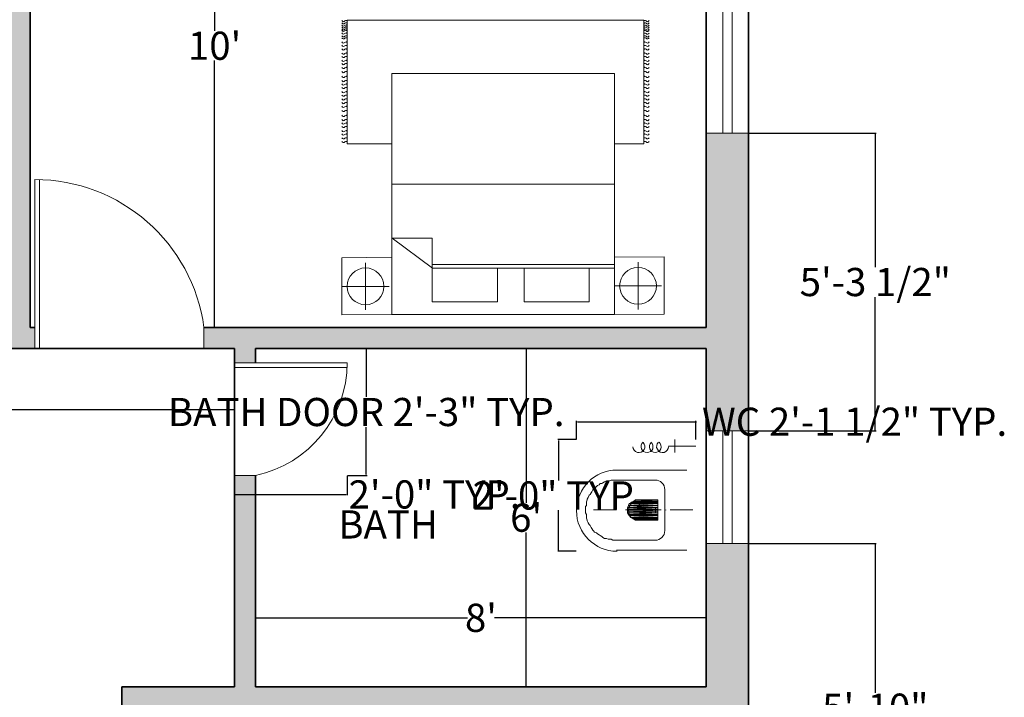
# Model space of a CAD drawing. Units: inches. Extents: x 302 to 1258, y 831 to 1373.
# Tile 12 of 13: x 1048 to 1258, y 1135 to 1279. Entities that reach past the tile are written whole.
import ezdxf

# ---------------------------------------------------------------- set-up
doc = ezdxf.new("R2010")
doc.units = ezdxf.units.IN
doc.header["$MEASUREMENT"] = 0
for name, color, linetype, lineweight in [('A-ANNO-DIMS', 2, 'Continuous', 18), ('A-AREA-IDEN', 7, 'Continuous', 18), ('A-DOOR', 3, 'Continuous', 18), ('A-FLOR-FIXT', 8, 'Continuous', 18), ('A-FURN', 8, 'Continuous', 18), ('A-GLAZ', 4, 'Continuous', 18), ('A-WALL', 7, 'Continuous', 35), ('A-WALL-PATT', 251, 'Continuous', 13)]:
    doc.layers.add(name, color=color, linetype=linetype, lineweight=lineweight)
doc.styles.get("Standard").update_dxf_attribs({"font": 'arial.ttf'})
doc.dimstyles.get("Standard").update_dxf_attribs({"dimtxt": 6, "dimasz": 0.18, "dimexe": 0.18, "dimexo": 0.0625, "dimgap": 0.09, "dimtad": 0, "dimtih": 1, "dimtoh": 1, "dimdec": 1, "dimzin": 0, "dimdsep": 46, "dimlunit": 3, "dimtxsty": 'Standard', "dimcen": 0.09, "dimadec": 0, "dimazin": 0, "dimtfac": 1, "dimtdec": 1, "dimtofl": 0, "dimtmove": 0, "dimatfit": 3, "dimfxl": 1, "dimtolj": 1, "dimtzin": 0, "dimarcsym": 0})

# ---------------------------------------------------------------- blocks, each defined once
blk = doc.blocks.new('*D22')
at = {"layer": 'A-ANNO-DIMS', "color": 0, "lineweight": -2, "transparency": 16777216}
for p, q in [((1194.06, 1333.32), (1089.21, 1333.32)), ((1089.39, 1333.14), (1089.39, 1276.47)), ((1089.39, 1213.5), (1089.39, 1270.17)), ((1194.06, 1213.32), (1089.21, 1213.32))]:
    blk.add_line(p, q, dxfattribs=at)
at = {"layer": 'A-ANNO-DIMS', "color": 0, "transparency": 16777216}
for points in [[(1089.36, 1333.14), (1089.42, 1333.14), (1089.39, 1333.32)], [(1089.36, 1213.5), (1089.42, 1213.5), (1089.39, 1213.32)]]:
    blk.add_solid(points, dxfattribs=at)
at = {"layer": 'Defpoints', "color": 0, "transparency": 16777216}
for p in [(1194.12, 1333.32), (1089.39, 1213.32), (1194.12, 1213.32)]:
    blk.add_point(p, dxfattribs=at)
at = {"layer": 'A-ANNO-DIMS', "color": 0, "transparency": 16777216, "insert": (1089.39, 1273.32), "char_height": 6, "attachment_point": 5}
blk.add_mtext("\\A1;10'", dxfattribs=at)
blk = doc.blocks.new('*D23')
at = {"layer": 'A-ANNO-DIMS', "color": 0, "lineweight": -2, "transparency": 16777216}
for p, q in [((1194.06, 1208.82), (1155.57, 1208.82)), ((1155.75, 1208.64), (1155.75, 1175.97)), ((1155.75, 1137), (1155.75, 1169.67)), ((1194.06, 1136.82), (1155.57, 1136.82))]:
    blk.add_line(p, q, dxfattribs=at)
at = {"layer": 'A-ANNO-DIMS', "color": 0, "transparency": 16777216}
for points in [[(1155.72, 1208.64), (1155.78, 1208.64), (1155.75, 1208.82)], [(1155.72, 1137), (1155.78, 1137), (1155.75, 1136.82)]]:
    blk.add_solid(points, dxfattribs=at)
at = {"layer": 'Defpoints', "color": 0, "transparency": 16777216}
for p in [(1155.75, 1208.82), (1194.12, 1208.82), (1194.12, 1136.82)]:
    blk.add_point(p, dxfattribs=at)
at = {"layer": 'A-ANNO-DIMS', "color": 0, "transparency": 16777216, "insert": (1155.75, 1172.82), "char_height": 6, "attachment_point": 5}
blk.add_mtext("\\A1;6'", dxfattribs=at)
blk = doc.blocks.new('*D24')
at = {"layer": 'A-ANNO-DIMS', "color": 0, "lineweight": -2, "transparency": 16777216}
for p, q in [((1098.12, 1136.88), (1098.12, 1151.68)), ((1098.3, 1151.5), (1143.27, 1151.5)), ((1193.94, 1151.5), (1148.98, 1151.5)), ((1194.12, 1136.88), (1194.12, 1151.68))]:
    blk.add_line(p, q, dxfattribs=at)
at = {"layer": 'A-ANNO-DIMS', "color": 0, "transparency": 16777216}
for points in [[(1098.3, 1151.53), (1098.3, 1151.47), (1098.12, 1151.5)], [(1193.94, 1151.53), (1193.94, 1151.47), (1194.12, 1151.5)]]:
    blk.add_solid(points, dxfattribs=at)
at = {"layer": 'Defpoints', "color": 0, "transparency": 16777216}
for p in [(1194.12, 1151.5), (1098.12, 1136.82), (1194.12, 1136.82)]:
    blk.add_point(p, dxfattribs=at)
at = {"layer": 'A-ANNO-DIMS', "color": 0, "transparency": 16777216, "insert": (1146.12, 1151.5), "char_height": 6, "attachment_point": 5}
blk.add_mtext("\\A1;8'", dxfattribs=at)
blk = doc.blocks.new('*D30')
at = {"layer": 'A-ANNO-DIMS', "color": 0, "lineweight": -2, "transparency": 16777216}
for p, q in [((937.62, 1208.76), (937.62, 1195.58)), ((1093.62, 1208.76), (1093.62, 1195.58)), ((937.8, 1195.76), (1010.72, 1195.76)), ((1093.44, 1195.76), (1020.52, 1195.76))]:
    blk.add_line(p, q, dxfattribs=at)
at = {"layer": 'A-ANNO-DIMS', "color": 0, "transparency": 16777216}
for points in [[(937.8, 1195.79), (937.8, 1195.73), (937.62, 1195.76)], [(1093.44, 1195.79), (1093.44, 1195.73), (1093.62, 1195.76)]]:
    blk.add_solid(points, dxfattribs=at)
at = {"layer": 'Defpoints', "color": 0, "transparency": 16777216}
for p in [(937.62, 1208.82), (1093.62, 1208.82), (1093.62, 1195.76)]:
    blk.add_point(p, dxfattribs=at)
at = {"layer": 'A-ANNO-DIMS', "color": 0, "transparency": 16777216, "insert": (1015.62, 1195.76), "char_height": 6, "attachment_point": 5}
blk.add_mtext("\\A1;13'", dxfattribs=at)
blk = doc.blocks.new('WC-PLAN')
h = blk.add_hatch(color=256)
h.paths.add_polyline_path([(17.3, 10.54), (11.83, 10.54), (17.3, 10.32)])
h.paths.add_polyline_path([(11.83, 10.54), (17.3, 10.32), (11.61, 10.32)])
h = blk.add_hatch(color=256)
h.paths.add_polyline_path([(17.3, 10.7), (12.21, 10.7), (17.3, 10.54)])
h.paths.add_polyline_path([(12.21, 10.7), (17.3, 10.54), (11.83, 10.54)])
h = blk.add_hatch(color=256)
h.paths.add_polyline_path([(17.3, 10.92), (12.59, 10.92), (17.3, 10.7)])
h.paths.add_polyline_path([(12.59, 10.92), (17.3, 10.7), (12.21, 10.7)])
h = blk.add_hatch(color=256)
h.paths.add_polyline_path([(17.3, 9.71), (11.08, 9.71), (17.3, 9.33)])
h.paths.add_polyline_path([(11.08, 9.71), (17.3, 9.33), (10.85, 9.33)])
h = blk.add_hatch(color=256)
h.paths.add_polyline_path([(17.3, 9.33), (10.85, 9.33), (17.3, 8.95)])
h.paths.add_polyline_path([(10.85, 9.33), (17.3, 8.95), (10.85, 8.95)])
h = blk.add_hatch(color=256)
h.paths.add_polyline_path([(17.3, 8.95), (10.85, 8.95), (17.3, 8.57)])
h.paths.add_polyline_path([(10.85, 8.95), (17.3, 8.57), (10.85, 8.57)])
h = blk.add_hatch(color=256)
h.paths.add_polyline_path([(17.3, 8.57), (10.85, 8.57), (17.3, 8.19)])
h.paths.add_polyline_path([(10.85, 8.57), (17.3, 8.19), (10.85, 8.19)])
h = blk.add_hatch(color=256)
h.paths.add_polyline_path([(17.3, 10.16), (11.23, 10.16), (17.3, 9.71)])
h.paths.add_polyline_path([(11.23, 10.16), (17.3, 9.71), (11.08, 9.71)])
h = blk.add_hatch(color=256)
h.paths.add_polyline_path([(17.3, 10.32), (11.61, 10.32), (17.3, 10.16)])
h.paths.add_polyline_path([(11.61, 10.32), (17.3, 10.16), (11.23, 10.16)])
h = blk.add_hatch(color=256)
h.paths.add_polyline_path([(17.3, 8.19), (10.85, 8.19), (17.3, 7.81)])
h.paths.add_polyline_path([(10.85, 8.19), (17.3, 7.81), (11.08, 7.81)])
h = blk.add_hatch(color=256)
h.paths.add_polyline_path([(17.3, 7.81), (11.08, 7.81), (17.3, 7.59)])
h.paths.add_polyline_path([(11.08, 7.81), (17.3, 7.59), (11.23, 7.59)])
h = blk.add_hatch(color=256)
h.paths.add_polyline_path([(17.3, 7.59), (11.23, 7.59), (17.3, 7.21)])
h.paths.add_polyline_path([(11.23, 7.59), (17.3, 7.21), (11.61, 7.21)])
h = blk.add_hatch(color=256)
h.paths.add_polyline_path([(17.3, 7.21), (11.61, 7.21), (17.3, 7.05)])
h.paths.add_polyline_path([(11.61, 7.21), (17.3, 7.05), (11.83, 7.05)])
h = blk.add_hatch(color=256)
h.paths.add_polyline_path([(17.3, 7.05), (11.83, 7.05), (17.3, 6.83)])
h.paths.add_polyline_path([(11.83, 7.05), (17.3, 6.83), (12.21, 6.83)])
h = blk.add_hatch(color=256)
h.paths.add_polyline_path([(17.3, 6.83), (12.21, 6.83), (17.3, 6.6)])
h.paths.add_polyline_path([(12.21, 6.83), (17.3, 6.6), (12.59, 6.6)])
h.paths.add_polyline_path([(17.3, 6.6), (12.59, 6.6), (12.97, 6.6)])
for points in [[(20.94, 21.03), (20.94, 23.77), (20.94, 23.77)], [(25.41, 22.4), (19.57, 22.4), (19.57, 22.4)], [(23.52, 17.3), (8.5, 17.3), (8.5, 17.3)], [(9.48, 2.35), (8.72, 2.35), (8.12, 2.35), (7.74, 2.35), (7.36, 2.58), (6.98, 2.58), (6.75, 2.58), (6.37, 2.73), (5.99, 2.73), (5.61, 2.96), (5.39, 3.11), (5.01, 3.34), (4.85, 3.49), (4.48, 3.72), (4.25, 3.94), (3.87, 4.1), (3.64, 4.32), (3.49, 4.48), (3.26, 4.85), (3.11, 5.08), (2.88, 5.46), (2.73, 5.69), (2.5, 6.07), (2.28, 6.45), (2.28, 6.6), (2.12, 7.05), (2.12, 7.43), (2.12, 7.81), (1.9, 8.19), (1.9, 8.8), (1.9, 9.56), (2.12, 9.71), (2.12, 10.16), (2.12, 10.54), (2.28, 10.92), (2.28, 11.07), (2.5, 11.45), (2.73, 11.91), (2.88, 12.06), (3.11, 12.44), (3.26, 12.67), (3.49, 13.05), (3.64, 13.2), (3.87, 13.43), (4.25, 13.81), (4.48, 14.03), (4.85, 14.18), (5.01, 14.41), (5.39, 14.41), (5.61, 14.56), (5.99, 14.79), (6.37, 15.02), (6.75, 15.02), (6.98, 15.02), (7.36, 15.17), (7.74, 15.17), (8.12, 15.17), (8.72, 15.17), (9.48, 15.17)], [(16.69, 15.17), (9.48, 15.17), (9.48, 15.17)], [(18.81, 4.48), (18.81, 13.2), (18.81, 13.2)], [(17.3, 10.92), (12.97, 10.92), (12.97, 10.92)], [(17.3, 6.6), (17.3, 10.92), (17.3, 10.92)], [(8.5, 8.8), (3.64, 8.8), (3.64, 8.8)], [(18.05, 8.8), (10.47, 8.8), (10.47, 8.8)], [(16.84, 9.18), (16.92, 9.18), (16.92, 9.18)], [(16.84, 8.8), (16.84, 8.95), (16.84, 9.18)], [(16.84, 8.8), (16.92, 8.72), (16.92, 8.72)], [(16.84, 8.34), (16.84, 8.57), (16.84, 8.8)], [(19.04, 8.8), (19.04, 8.72), (19.04, 8.72)], [(24.81, 8.8), (19.95, 8.8), (19.95, 8.8)], [(17.3, 6.6), (12.97, 6.6), (12.97, 6.6)], [(16.84, 8.34), (16.92, 8.34), (16.92, 8.34)], [(16.69, 2.35), (9.48, 2.35), (9.48, 2.35)], [(23.52, 0.23), (8.5, 0.23), (8.5, 0.23)]]:
    blk.add_lwpolyline(points)
for points in [[(11.83, 10.54), (17.3, 10.32), (11.61, 10.32)], [(12.21, 10.7), (17.3, 10.54), (11.83, 10.54)], [(17.3, 10.54), (11.83, 10.54), (17.3, 10.32)], [(12.59, 10.92), (17.3, 10.7), (12.21, 10.7)], [(17.3, 10.7), (12.21, 10.7), (17.3, 10.54)], [(12.97, 10.92), (17.3, 10.92), (12.59, 10.92)], [(17.3, 10.92), (12.59, 10.92), (17.3, 10.7)], [(17.3, 10.92), (12.97, 10.92)], [(11.08, 9.71), (17.3, 9.33), (10.85, 9.33)], [(17.3, 9.33), (10.85, 9.33), (17.3, 8.95)], [(10.85, 9.33), (17.3, 8.95), (10.85, 8.95)], [(17.3, 8.95), (10.85, 8.95), (17.3, 8.57)], [(10.85, 8.95), (17.3, 8.57), (10.85, 8.57)], [(17.3, 8.57), (10.85, 8.57), (17.3, 8.19)], [(10.85, 8.57), (17.3, 8.19), (10.85, 8.19)], [(11.23, 10.16), (17.3, 9.71), (11.08, 9.71)], [(17.3, 9.71), (11.08, 9.71), (17.3, 9.33)], [(11.61, 10.32), (17.3, 10.16), (11.23, 10.16)], [(17.3, 10.16), (11.23, 10.16), (17.3, 9.71)], [(17.3, 10.32), (11.61, 10.32), (17.3, 10.16)], [(17.3, 8.19), (10.85, 8.19), (17.3, 7.81)], [(10.85, 8.19), (17.3, 7.81), (11.08, 7.81)], [(17.3, 7.81), (11.08, 7.81), (17.3, 7.59)], [(11.08, 7.81), (17.3, 7.59), (11.23, 7.59)], [(17.3, 7.59), (11.23, 7.59), (17.3, 7.21)], [(11.23, 7.59), (17.3, 7.21), (11.61, 7.21)], [(17.3, 7.21), (11.61, 7.21), (17.3, 7.05)], [(11.61, 7.21), (17.3, 7.05), (11.83, 7.05)], [(17.3, 7.05), (11.83, 7.05), (17.3, 6.83)], [(11.83, 7.05), (17.3, 6.83), (12.21, 6.83)], [(17.3, 6.83), (12.21, 6.83), (17.3, 6.6)], [(12.21, 6.83), (17.3, 6.6), (12.59, 6.6)], [(17.3, 6.6), (12.59, 6.6), (12.97, 6.6)], [(12.59, 6.6), (17.3, 6.6), (17.3, 6.6)]]:
    blk.add_lwpolyline(points, close=True)
for points, knots in [([(11.99, 22.25), (11.99, 21.72), (12.44, 21.19), (12.97, 21.03), (12.97, 21.03), (13.5, 20.88), (14.11, 21.19), (14.41, 21.64), (14.41, 21.64), (14.64, 22.17), (14.56, 22.78), (14.19, 23.16)], [0, 0, 0, 0, 0.083333, 0.083333, 0.083333, 0.083334, 0.166667, 0.166667, 0.166667, 0.166668, 1, 1, 1, 1]), ([(14.19, 23.23), (13.81, 22.86), (13.65, 22.32), (13.88, 21.79), (13.88, 21.79), (14.03, 21.34), (14.49, 21.03), (15.02, 21.03), (15.02, 21.03), (15.55, 21.03), (16.01, 21.34), (16.23, 21.79), (16.23, 21.79), (16.39, 22.32), (16.23, 22.86), (15.85, 23.23)], [0, 0, 0, 0, 0.0625, 0.0625, 0.0625, 0.062501, 0.125, 0.125, 0.125, 0.125001, 0.1875, 0.1875, 0.1875, 0.187501, 1, 1, 1, 1]), ([(15.93, 23.16), (15.55, 22.86), (15.4, 22.25), (15.63, 21.79), (15.63, 21.79), (15.78, 21.34), (16.31, 21.03), (16.76, 21.03), (16.76, 21.03), (17.3, 21.03), (17.75, 21.34), (17.98, 21.79), (17.98, 21.79), (18.13, 22.32), (17.98, 22.86), (17.6, 23.23)], [0, 0, 0, 0, 0.0625, 0.0625, 0.0625, 0.062501, 0.125, 0.125, 0.125, 0.125001, 0.1875, 0.1875, 0.1875, 0.187501, 1, 1, 1, 1]), ([(17.45, 23.23), (17.07, 22.86), (16.92, 22.17), (17.22, 21.72), (17.22, 21.72), (17.52, 21.19), (18.05, 20.88), (18.66, 21.03), (18.66, 21.03), (19.19, 21.19), (19.57, 21.72), (19.57, 22.25)], [0, 0, 0, 0, 0.083333, 0.083333, 0.083333, 0.083334, 0.166667, 0.166667, 0.166667, 0.166668, 1, 1, 1, 1]), ([(8.65, 17.3), (3.87, 17.3), (0, 13.43), (0, 8.65), (0, 8.65), (0, 3.87), (3.87, 0), (8.65, 0)], [0, 0, 0, 0, 0.125, 0.125, 0.125, 0.125001, 1, 1, 1, 1]), ([(13.12, 10.7), (11.99, 10.7), (11.08, 9.79), (11.08, 8.65), (11.08, 8.65), (11.08, 7.51), (11.99, 6.6), (13.12, 6.6)], [0, 0, 0, 0, 0.125, 0.125, 0.125, 0.125001, 1, 1, 1, 1])]:
    blk.add_open_spline(points, degree=3, knots=knots)
for points in [[(18.81, 13.12), (18.81, 14.26), (17.9, 15.17), (16.76, 15.17)], [(16.76, 2.35), (17.9, 2.35), (18.81, 3.26), (18.81, 4.4)]]:
    blk.add_open_spline(points, degree=3)
blk = doc.blocks.new('BED-DOUBLE-WITH-NIGHTSTANDS')
for p, q in [((1.12, 36.41), (1.12, 62.78)), ((1.12, 62.78), (64.36, 62.78)), ((64.36, 62.78), (64.36, 36.41)), ((10.66, 36.41), (1.12, 36.41)), ((64.36, 36.41), (58.06, 36.41)), ((10.66, 27.82), (58.08, 27.82)), ((19.27, 16.32), (10.71, 16.32)), ((19.32, 9.97), (10.71, 16.32)), ((19.27, 9.97), (19.27, 16.32)), ((5.06, 1.07), (5.06, 11.12)), ((19.27, 10.78), (58.08, 10.78)), ((63.11, 1.17), (63.11, 11.22)), ((19.32, 9.97), (58.08, 9.97)), ((0.03, 6.09), (10.09, 6.09)), ((58.08, 6.2), (68.14, 6.2))]:
    blk.add_line(p, q)
for points in [[(10.66, 0.1), (10.66, 51.42), (58.08, 51.42), (58.08, 0.1)], [(10.66, 12.29), (0.03, 12.19), (0.03, 0), (10.66, 0.1)], [(68.71, 12.39), (58.08, 12.29), (58.08, 0.1), (68.71, 0.2)], [(19.27, 2.8), (19.27, 9.97), (33.16, 9.97), (33.16, 2.8)], [(38.83, 2.8), (38.83, 9.97), (52.73, 9.97), (52.73, 2.8)]]:
    blk.add_lwpolyline(points, close=True)
for centre in [(5.06, 6.09), (63.11, 6.2)]:
    blk.add_circle(centre, 3.92)
for points, knots in [([(0, 62.71), (0.1, 62.59), (0.29, 62.35), (0.63, 62.59), (0.91, 62.76), (1.06, 62.66), (1.13, 62.61)], [0, 0, 0, 0, 0.400747, 0.791423, 1.067667, 1.29709, 1.29709, 1.29709, 1.29709]), ([(0, 62.24), (0.1, 62.12), (0.29, 61.88), (0.63, 62.12), (0.91, 62.29), (1.06, 62.18), (1.13, 62.13)], [0, 0, 0, 0, 0.400747, 0.791423, 1.067667, 1.29709, 1.29709, 1.29709, 1.29709]), ([(0, 61.75), (0.1, 61.63), (0.29, 61.39), (0.63, 61.63), (0.91, 61.8), (1.06, 61.7), (1.13, 61.65)], [0, 0, 0, 0, 0.400747, 0.791423, 1.067667, 1.29709, 1.29709, 1.29709, 1.29709]), ([(0, 61.35), (0.1, 61.23), (0.29, 60.99), (0.63, 61.23), (0.91, 61.41), (1.06, 61.3), (1.13, 61.25)], [0, 0, 0, 0, 0.400747, 0.791423, 1.067667, 1.29709, 1.29709, 1.29709, 1.29709]), ([(0, 60.94), (0.1, 60.81), (0.29, 60.58), (0.63, 60.81), (0.91, 60.99), (1.05, 60.89), (1.12, 60.84)], [0, 0, 0, 0, 0.400747, 0.791423, 1.067667, 1.283686, 1.283686, 1.283686, 1.283686]), ([(65.48, 62.71), (65.39, 62.59), (65.19, 62.35), (64.85, 62.59), (64.57, 62.76), (64.42, 62.66), (64.36, 62.61)], [0, 0, 0, 0, 0.400747, 0.791423, 1.067667, 1.29709, 1.29709, 1.29709, 1.29709]), ([(65.48, 62.21), (65.39, 62.09), (65.19, 61.85), (64.85, 62.09), (64.57, 62.26), (64.42, 62.15), (64.36, 62.11)], [0, 0, 0, 0, 0.400747, 0.791423, 1.067667, 1.29709, 1.29709, 1.29709, 1.29709]), ([(65.48, 61.72), (65.39, 61.6), (65.19, 61.36), (64.85, 61.6), (64.57, 61.78), (64.42, 61.67), (64.36, 61.62)], [0, 0, 0, 0, 0.400747, 0.791423, 1.067667, 1.29709, 1.29709, 1.29709, 1.29709]), ([(65.48, 61.33), (65.39, 61.21), (65.19, 60.97), (64.85, 61.21), (64.57, 61.38), (64.42, 61.27), (64.36, 61.22)], [0, 0, 0, 0, 0.400747, 0.791423, 1.067667, 1.29709, 1.29709, 1.29709, 1.29709]), ([(65.48, 60.91), (65.39, 60.79), (65.19, 60.55), (64.85, 60.79), (64.57, 60.96), (64.42, 60.85), (64.36, 60.81)], [0, 0, 0, 0, 0.400747, 0.791423, 1.067667, 1.29709, 1.29709, 1.29709, 1.29709]), ([(0, 60.63), (0.1, 60.51), (0.29, 60.27), (0.63, 60.51), (0.91, 60.68), (1.05, 60.58), (1.12, 60.53)], [0, 0, 0, 0, 0.400747, 0.791423, 1.067667, 1.283686, 1.283686, 1.283686, 1.283686]), ([(0, 60.05), (0.1, 59.93), (0.29, 59.69), (0.63, 59.93), (0.91, 60.1), (1.05, 60), (1.12, 59.96)], [0, 0, 0, 0, 0.400747, 0.791423, 1.067667, 1.283686, 1.283686, 1.283686, 1.283686]), ([(0, 59.46), (0.1, 59.34), (0.29, 59.09), (0.63, 59.34), (0.91, 59.51), (1.05, 59.41), (1.12, 59.36)], [0, 0, 0, 0, 0.402903, 0.794912, 1.071156, 1.287177, 1.287177, 1.287177, 1.287177]), ([(0, 59.03), (0.1, 58.91), (0.29, 58.67), (0.63, 58.91), (0.91, 59.08), (1.05, 58.98), (1.12, 58.93)], [0, 0, 0, 0, 0.400747, 0.791423, 1.067667, 1.283686, 1.283686, 1.283686, 1.283686]), ([(65.48, 60.6), (65.39, 60.48), (65.19, 60.24), (64.85, 60.48), (64.57, 60.65), (64.42, 60.54), (64.36, 60.5)], [0, 0, 0, 0, 0.400747, 0.791423, 1.067667, 1.29709, 1.29709, 1.29709, 1.29709]), ([(65.48, 60.03), (65.39, 59.9), (65.19, 59.67), (64.85, 59.9), (64.57, 60.08), (64.42, 59.97), (64.36, 59.92)], [0, 0, 0, 0, 0.400747, 0.791423, 1.067667, 1.29709, 1.29709, 1.29709, 1.29709]), ([(65.48, 59.46), (65.39, 59.33), (65.2, 59.08), (64.85, 59.34), (64.57, 59.51), (64.42, 59.4), (64.36, 59.36)], [0, 0, 0, 0, 0.407265, 0.802015, 1.07826, 1.307683, 1.307683, 1.307683, 1.307683]), ([(65.48, 59.03), (65.39, 58.91), (65.19, 58.67), (64.85, 58.91), (64.57, 59.08), (64.42, 58.97), (64.36, 58.93)], [0, 0, 0, 0, 0.400747, 0.791423, 1.067667, 1.29709, 1.29709, 1.29709, 1.29709]), ([(0, 58.15), (0.1, 58.03), (0.29, 57.79), (0.63, 58.03), (0.91, 58.2), (1.05, 58.1), (1.12, 58.05)], [0, 0, 0, 0, 0.400747, 0.791423, 1.067667, 1.283686, 1.283686, 1.283686, 1.283686]), ([(0, 57.42), (0.1, 57.3), (0.29, 57.06), (0.63, 57.3), (0.91, 57.47), (1.06, 57.36), (1.13, 57.32)], [0, 0, 0, 0, 0.400747, 0.791423, 1.067667, 1.29709, 1.29709, 1.29709, 1.29709]), ([(0, 56.67), (0.1, 56.55), (0.29, 56.31), (0.63, 56.55), (0.91, 56.72), (1.06, 56.61), (1.13, 56.56)], [0, 0, 0, 0, 0.400747, 0.791423, 1.067667, 1.29709, 1.29709, 1.29709, 1.29709]), ([(65.48, 58.15), (65.39, 58.03), (65.19, 57.79), (64.85, 58.03), (64.57, 58.2), (64.42, 58.09), (64.36, 58.04)], [0, 0, 0, 0, 0.400747, 0.791423, 1.067667, 1.29709, 1.29709, 1.29709, 1.29709]), ([(65.48, 57.42), (65.39, 57.3), (65.19, 57.06), (64.85, 57.3), (64.57, 57.47), (64.42, 57.36), (64.36, 57.32)], [0, 0, 0, 0, 0.400747, 0.791423, 1.067667, 1.29709, 1.29709, 1.29709, 1.29709]), ([(65.48, 56.67), (65.39, 56.55), (65.19, 56.31), (64.85, 56.55), (64.57, 56.72), (64.42, 56.61), (64.36, 56.56)], [0, 0, 0, 0, 0.400747, 0.791423, 1.067667, 1.29709, 1.29709, 1.29709, 1.29709]), ([(0, 55.78), (0.1, 55.66), (0.29, 55.42), (0.63, 55.66), (0.91, 55.84), (1.06, 55.73), (1.13, 55.68)], [0, 0, 0, 0, 0.400747, 0.791423, 1.067667, 1.29709, 1.29709, 1.29709, 1.29709]), ([(0, 55.06), (0.1, 54.94), (0.29, 54.7), (0.63, 54.94), (0.91, 55.11), (1.06, 55), (1.13, 54.95)], [0, 0, 0, 0, 0.400747, 0.791423, 1.067667, 1.29709, 1.29709, 1.29709, 1.29709]), ([(65.48, 55.78), (65.39, 55.66), (65.19, 55.42), (64.85, 55.66), (64.57, 55.84), (64.42, 55.73), (64.36, 55.68)], [0, 0, 0, 0, 0.400747, 0.791423, 1.067667, 1.29709, 1.29709, 1.29709, 1.29709]), ([(65.48, 55.06), (65.39, 54.94), (65.19, 54.7), (64.85, 54.94), (64.57, 55.11), (64.42, 55), (64.36, 54.95)], [0, 0, 0, 0, 0.400747, 0.791423, 1.067667, 1.29709, 1.29709, 1.29709, 1.29709]), ([(0, 54.24), (0.1, 54.12), (0.29, 53.88), (0.63, 54.12), (0.91, 54.29), (1.06, 54.19), (1.13, 54.14)], [0, 0, 0, 0, 0.400747, 0.791423, 1.067667, 1.29709, 1.29709, 1.29709, 1.29709]), ([(0, 53.55), (0.1, 53.43), (0.29, 53.19), (0.63, 53.43), (0.91, 53.6), (1.06, 53.5), (1.13, 53.45)], [0, 0, 0, 0, 0.400747, 0.791423, 1.067667, 1.29709, 1.29709, 1.29709, 1.29709]), ([(0, 52.73), (0.1, 52.61), (0.29, 52.37), (0.63, 52.61), (0.91, 52.79), (1.06, 52.68), (1.13, 52.63)], [0, 0, 0, 0, 0.400747, 0.791423, 1.067667, 1.29709, 1.29709, 1.29709, 1.29709]), ([(65.48, 54.24), (65.39, 54.12), (65.19, 53.88), (64.85, 54.12), (64.57, 54.29), (64.42, 54.19), (64.36, 54.14)], [0, 0, 0, 0, 0.400747, 0.791423, 1.067667, 1.29709, 1.29709, 1.29709, 1.29709]), ([(65.48, 53.55), (65.39, 53.43), (65.19, 53.19), (64.85, 53.43), (64.57, 53.6), (64.42, 53.5), (64.36, 53.45)], [0, 0, 0, 0, 0.400747, 0.791423, 1.067667, 1.29709, 1.29709, 1.29709, 1.29709]), ([(65.48, 52.73), (65.39, 52.61), (65.19, 52.37), (64.85, 52.61), (64.57, 52.79), (64.42, 52.68), (64.36, 52.63)], [0, 0, 0, 0, 0.400747, 0.791423, 1.067667, 1.29709, 1.29709, 1.29709, 1.29709]), ([(0, 51.85), (0.1, 51.73), (0.29, 51.49), (0.63, 51.73), (0.91, 51.9), (1.06, 51.8), (1.13, 51.75)], [0, 0, 0, 0, 0.400747, 0.791423, 1.067667, 1.29709, 1.29709, 1.29709, 1.29709]), ([(0, 50.82), (0.1, 50.69), (0.29, 50.46), (0.63, 50.69), (0.91, 50.87), (1.06, 50.76), (1.13, 50.71)], [0, 0, 0, 0, 0.400747, 0.791423, 1.067667, 1.29709, 1.29709, 1.29709, 1.29709]), ([(65.48, 51.85), (65.39, 51.73), (65.19, 51.49), (64.85, 51.73), (64.57, 51.9), (64.42, 51.8), (64.36, 51.75)], [0, 0, 0, 0, 0.400747, 0.791423, 1.067667, 1.29709, 1.29709, 1.29709, 1.29709]), ([(65.48, 50.82), (65.39, 50.69), (65.19, 50.46), (64.85, 50.69), (64.57, 50.87), (64.42, 50.76), (64.36, 50.71)], [0, 0, 0, 0, 0.400747, 0.791423, 1.067667, 1.29709, 1.29709, 1.29709, 1.29709]), ([(0, 49.93), (0.1, 49.81), (0.29, 49.57), (0.63, 49.81), (0.91, 49.99), (1.06, 49.88), (1.13, 49.83)], [0, 0, 0, 0, 0.400747, 0.791423, 1.067667, 1.29709, 1.29709, 1.29709, 1.29709]), ([(0, 49.21), (0.1, 49.08), (0.29, 48.84), (0.63, 49.08), (0.91, 49.26), (1.06, 49.15), (1.13, 49.1)], [0, 0, 0, 0, 0.400747, 0.791423, 1.067667, 1.29709, 1.29709, 1.29709, 1.29709]), ([(0, 48.45), (0.1, 48.33), (0.29, 48.09), (0.63, 48.33), (0.91, 48.51), (1.06, 48.4), (1.13, 48.35)], [0, 0, 0, 0, 0.400747, 0.791423, 1.067667, 1.29709, 1.29709, 1.29709, 1.29709]), ([(65.48, 49.93), (65.39, 49.81), (65.19, 49.57), (64.85, 49.81), (64.57, 49.99), (64.42, 49.88), (64.36, 49.83)], [0, 0, 0, 0, 0.400747, 0.791423, 1.067667, 1.29709, 1.29709, 1.29709, 1.29709]), ([(65.48, 49.21), (65.39, 49.08), (65.19, 48.84), (64.85, 49.08), (64.57, 49.26), (64.42, 49.15), (64.36, 49.1)], [0, 0, 0, 0, 0.400747, 0.791423, 1.067667, 1.29709, 1.29709, 1.29709, 1.29709]), ([(65.48, 48.45), (65.39, 48.33), (65.19, 48.09), (64.85, 48.33), (64.57, 48.51), (64.42, 48.4), (64.36, 48.35)], [0, 0, 0, 0, 0.400747, 0.791423, 1.067667, 1.29709, 1.29709, 1.29709, 1.29709]), ([(0, 47.57), (0.1, 47.45), (0.29, 47.21), (0.63, 47.45), (0.91, 47.62), (1.06, 47.52), (1.13, 47.47)], [0, 0, 0, 0, 0.400747, 0.791423, 1.067667, 1.29709, 1.29709, 1.29709, 1.29709]), ([(0, 46.84), (0.1, 46.72), (0.29, 46.48), (0.63, 46.72), (0.91, 46.89), (1.06, 46.79), (1.13, 46.74)], [0, 0, 0, 0, 0.400747, 0.791423, 1.067667, 1.29709, 1.29709, 1.29709, 1.29709]), ([(65.48, 47.57), (65.39, 47.45), (65.19, 47.21), (64.85, 47.45), (64.57, 47.62), (64.42, 47.52), (64.36, 47.47)], [0, 0, 0, 0, 0.400747, 0.791423, 1.067667, 1.29709, 1.29709, 1.29709, 1.29709]), ([(65.48, 46.84), (65.39, 46.72), (65.19, 46.48), (64.85, 46.72), (64.57, 46.89), (64.42, 46.79), (64.36, 46.74)], [0, 0, 0, 0, 0.400747, 0.791423, 1.067667, 1.29709, 1.29709, 1.29709, 1.29709]), ([(0, 46.03), (0.1, 45.91), (0.29, 45.67), (0.63, 45.91), (0.91, 46.08), (1.06, 45.97), (1.13, 45.92)], [0, 0, 0, 0, 0.400747, 0.791423, 1.067667, 1.29709, 1.29709, 1.29709, 1.29709]), ([(0, 45.25), (0.1, 45.13), (0.29, 44.89), (0.63, 45.13), (0.91, 45.3), (1.06, 45.2), (1.13, 45.15)], [0, 0, 0, 0, 0.400747, 0.791423, 1.067667, 1.29709, 1.29709, 1.29709, 1.29709]), ([(0, 44.43), (0.1, 44.31), (0.29, 44.07), (0.63, 44.31), (0.91, 44.49), (1.06, 44.38), (1.13, 44.33)], [0, 0, 0, 0, 0.400747, 0.791423, 1.067667, 1.29709, 1.29709, 1.29709, 1.29709]), ([(65.48, 46.03), (65.39, 45.91), (65.19, 45.67), (64.85, 45.91), (64.57, 46.08), (64.42, 45.97), (64.36, 45.92)], [0, 0, 0, 0, 0.400747, 0.791423, 1.067667, 1.29709, 1.29709, 1.29709, 1.29709]), ([(65.48, 45.25), (65.39, 45.13), (65.19, 44.89), (64.85, 45.13), (64.57, 45.3), (64.42, 45.2), (64.36, 45.15)], [0, 0, 0, 0, 0.400747, 0.791423, 1.067667, 1.29709, 1.29709, 1.29709, 1.29709]), ([(65.48, 44.43), (65.39, 44.31), (65.19, 44.07), (64.85, 44.31), (64.57, 44.49), (64.42, 44.38), (64.36, 44.33)], [0, 0, 0, 0, 0.400747, 0.791423, 1.067667, 1.29709, 1.29709, 1.29709, 1.29709]), ([(0, 43.55), (0.1, 43.43), (0.29, 43.19), (0.63, 43.43), (0.91, 43.6), (1.06, 43.5), (1.13, 43.45)], [0, 0, 0, 0, 0.400747, 0.791423, 1.067667, 1.29709, 1.29709, 1.29709, 1.29709]), ([(0, 42.52), (0.1, 42.39), (0.29, 42.15), (0.63, 42.39), (0.91, 42.57), (1.06, 42.46), (1.13, 42.41)], [0, 0, 0, 0, 0.400747, 0.791423, 1.067667, 1.29709, 1.29709, 1.29709, 1.29709]), ([(65.48, 43.55), (65.39, 43.43), (65.19, 43.19), (64.85, 43.43), (64.57, 43.6), (64.42, 43.5), (64.36, 43.45)], [0, 0, 0, 0, 0.400747, 0.791423, 1.067667, 1.29709, 1.29709, 1.29709, 1.29709]), ([(65.48, 42.52), (65.39, 42.39), (65.19, 42.15), (64.85, 42.39), (64.57, 42.57), (64.42, 42.46), (64.36, 42.41)], [0, 0, 0, 0, 0.400747, 0.791423, 1.067667, 1.29709, 1.29709, 1.29709, 1.29709]), ([(0, 41.63), (0.1, 41.51), (0.29, 41.27), (0.63, 41.51), (0.91, 41.68), (1.06, 41.58), (1.13, 41.53)], [0, 0, 0, 0, 0.400747, 0.791423, 1.067667, 1.29709, 1.29709, 1.29709, 1.29709]), ([(0, 40.9), (0.1, 40.78), (0.29, 40.54), (0.63, 40.78), (0.91, 40.96), (1.06, 40.85), (1.13, 40.8)], [0, 0, 0, 0, 0.400747, 0.791423, 1.067667, 1.29709, 1.29709, 1.29709, 1.29709]), ([(0, 40.15), (0.1, 40.03), (0.29, 39.79), (0.63, 40.03), (0.91, 40.2), (1.06, 40.1), (1.13, 40.05)], [0, 0, 0, 0, 0.400747, 0.791423, 1.067667, 1.29709, 1.29709, 1.29709, 1.29709]), ([(65.48, 41.63), (65.39, 41.51), (65.19, 41.27), (64.85, 41.51), (64.57, 41.68), (64.42, 41.58), (64.36, 41.53)], [0, 0, 0, 0, 0.400747, 0.791423, 1.067667, 1.29709, 1.29709, 1.29709, 1.29709]), ([(65.48, 40.9), (65.39, 40.78), (65.19, 40.54), (64.85, 40.78), (64.57, 40.96), (64.42, 40.85), (64.36, 40.8)], [0, 0, 0, 0, 0.400747, 0.791423, 1.067667, 1.29709, 1.29709, 1.29709, 1.29709]), ([(65.48, 40.15), (65.39, 40.03), (65.19, 39.79), (64.85, 40.03), (64.57, 40.2), (64.42, 40.1), (64.36, 40.05)], [0, 0, 0, 0, 0.400747, 0.791423, 1.067667, 1.29709, 1.29709, 1.29709, 1.29709]), ([(0, 39.27), (0.1, 39.15), (0.29, 38.91), (0.63, 39.15), (0.91, 39.32), (1.06, 39.22), (1.13, 39.17)], [0, 0, 0, 0, 0.400747, 0.791423, 1.067667, 1.29709, 1.29709, 1.29709, 1.29709]), ([(0, 38.54), (0.1, 38.42), (0.29, 38.18), (0.63, 38.42), (0.91, 38.59), (1.06, 38.49), (1.13, 38.44)], [0, 0, 0, 0, 0.400747, 0.791423, 1.067667, 1.29709, 1.29709, 1.29709, 1.29709]), ([(65.48, 39.27), (65.39, 39.15), (65.19, 38.91), (64.85, 39.15), (64.57, 39.32), (64.42, 39.22), (64.36, 39.17)], [0, 0, 0, 0, 0.400747, 0.791423, 1.067667, 1.29709, 1.29709, 1.29709, 1.29709]), ([(65.48, 38.54), (65.39, 38.42), (65.19, 38.18), (64.85, 38.42), (64.57, 38.59), (64.42, 38.49), (64.36, 38.44)], [0, 0, 0, 0, 0.400747, 0.791423, 1.067667, 1.29709, 1.29709, 1.29709, 1.29709]), ([(0, 37.73), (0.1, 37.61), (0.29, 37.37), (0.63, 37.61), (0.91, 37.78), (1.06, 37.67), (1.13, 37.62)], [0, 0, 0, 0, 0.400747, 0.791423, 1.067667, 1.29709, 1.29709, 1.29709, 1.29709]), ([(0, 36.95), (0.1, 36.83), (0.29, 36.59), (0.63, 36.83), (0.91, 37), (1.06, 36.89), (1.13, 36.85)], [0, 0, 0, 0, 0.400747, 0.791423, 1.067667, 1.29709, 1.29709, 1.29709, 1.29709]), ([(65.48, 37.73), (65.39, 37.61), (65.19, 37.37), (64.85, 37.61), (64.57, 37.78), (64.42, 37.67), (64.36, 37.62)], [0, 0, 0, 0, 0.400747, 0.791423, 1.067667, 1.29709, 1.29709, 1.29709, 1.29709]), ([(65.48, 36.95), (65.39, 36.83), (65.19, 36.59), (64.85, 36.83), (64.57, 37), (64.42, 36.89), (64.36, 36.85)], [0, 0, 0, 0, 0.400747, 0.791423, 1.067667, 1.29709, 1.29709, 1.29709, 1.29709])]:
    blk.add_open_spline(points, degree=3, knots=knots)
blk = doc.blocks.new('WINDOW-48IN')
for p, q in [((0, 0), (0, 9)), ((0, 9), (48, 9)), ((48, 9), (48, 0)), ((0, 5.5), (48, 5.5)), ((48, 3.5), (0, 3.5)), ((48, 0), (0, 0))]:
    blk.add_line(p, q)
blk = doc.blocks.new('VENT-WINDOW-24IN')
for p, q in [((0, 24), (9, 24)), ((0, 0), (0, 24)), ((3.5, 0), (3.5, 24)), ((5.5, 24), (5.5, 0)), ((9, 24), (9, 0)), ((9, 0), (0, 0))]:
    blk.add_line(p, q)
blk = doc.blocks.new('DOOR-36IN-BEDROOM')
for p, q in [((35, 36), (35, 0)), ((36, 0), (36, 36)), ((36, 36), (36, 0)), ((0, 0), (0, 4.5)), ((36, 0), (0, 0)), ((37, 0), (36, 0))]:
    blk.add_line(p, q)
blk.add_arc((36, -0.32), 36.32, 90, 172.3719)
blk = doc.blocks.new('DOOR-24IN-BATH')
for p, q in [((0, 27), (0, 24)), ((0, 24), (24, 24)), ((24, 24), (0, 24)), ((0, 24), (0, 0)), ((24, 23), (0, 23)), ((0, 0), (4.5, 0))]:
    blk.add_line(p, q)
blk.add_arc((-0.52, 24), 24.52, 281.8123, 0)
blk = doc.blocks.new('*D49')
at = {"layer": 'A-ANNO-DIMS', "color": 0, "lineweight": -2, "transparency": 16777216}
for p, q in [((1166.47, 1189.5), (1166.47, 1193.43)), ((1191.88, 1189.5), (1191.88, 1193.43)), ((1166.65, 1193.25), (1191.7, 1193.25)), ((1191.88, 1193.25), (1192.06, 1193.25))]:
    blk.add_line(p, q, dxfattribs=at)
at = {"layer": 'A-ANNO-DIMS', "color": 0, "transparency": 16777216}
for points in [[(1166.65, 1193.28), (1166.65, 1193.22), (1166.47, 1193.25)], [(1191.7, 1193.28), (1191.7, 1193.22), (1191.88, 1193.25)]]:
    blk.add_solid(points, dxfattribs=at)
at = {"layer": 'Defpoints', "color": 0, "transparency": 16777216}
for p in [(1191.88, 1193.25), (1166.47, 1189.44), (1191.88, 1189.44)]:
    blk.add_point(p, dxfattribs=at)
at = {"layer": 'A-ANNO-DIMS', "color": 0, "transparency": 16777216, "insert": (1225.7, 1193.25), "char_height": 6, "attachment_point": 5}
blk.add_mtext('\\A1;WC 2\'-1 1/2" TYP.', dxfattribs=at)
blk = doc.blocks.new('*D50')
at = {"layer": 'A-ANNO-DIMS', "color": 0, "lineweight": -2, "transparency": 16777216}
for p, q in [((1166.4, 1189.44), (1162.48, 1189.44)), ((1162.66, 1189.26), (1162.66, 1180.71)), ((1162.66, 1165.85), (1162.66, 1174.4)), ((1166.4, 1165.67), (1162.48, 1165.67))]:
    blk.add_line(p, q, dxfattribs=at)
at = {"layer": 'A-ANNO-DIMS', "color": 0, "transparency": 16777216}
for points in [[(1162.63, 1189.26), (1162.69, 1189.26), (1162.66, 1189.44)], [(1162.63, 1165.85), (1162.69, 1165.85), (1162.66, 1165.67)]]:
    blk.add_solid(points, dxfattribs=at)
at = {"layer": 'Defpoints', "color": 0, "transparency": 16777216}
for p in [(1162.66, 1189.44), (1166.47, 1189.44), (1166.47, 1165.67)]:
    blk.add_point(p, dxfattribs=at)
at = {"layer": 'A-ANNO-DIMS', "color": 0, "transparency": 16777216, "insert": (1162.66, 1177.55), "char_height": 6, "attachment_point": 5}
blk.add_mtext('\\A1;2\'-0" TYP.', dxfattribs=at)
blk = doc.blocks.new('*D57')
at = {"layer": 'A-ANNO-DIMS', "color": 0, "lineweight": -2, "transparency": 16777216}
for p, q in [((1117.68, 1208.82), (1121.85, 1208.82)), ((1121.67, 1208.64), (1121.67, 1198.52)), ((1121.67, 1182), (1121.67, 1192.12)), ((1117.68, 1181.82), (1121.85, 1181.82))]:
    blk.add_line(p, q, dxfattribs=at)
at = {"layer": 'A-ANNO-DIMS', "color": 0, "transparency": 16777216}
for points in [[(1121.64, 1208.64), (1121.7, 1208.64), (1121.67, 1208.82)], [(1121.64, 1182), (1121.7, 1182), (1121.67, 1181.82)]]:
    blk.add_solid(points, dxfattribs=at)
at = {"layer": 'Defpoints', "color": 0, "transparency": 16777216}
for p in [(1117.62, 1208.82), (1121.67, 1208.82), (1117.62, 1181.82)]:
    blk.add_point(p, dxfattribs=at)
at = {"layer": 'A-ANNO-DIMS', "color": 0, "transparency": 16777216, "insert": (1121.67, 1195.32), "char_height": 6, "attachment_point": 5}
blk.add_mtext('\\A1;BATH DOOR 2\'-3" TYP.', dxfattribs=at)
blk = doc.blocks.new('*D58')
at = {"layer": 'A-ANNO-DIMS', "color": 0, "lineweight": -2, "transparency": 16777216}
for p, q in [((1093.62, 1181.76), (1093.62, 1177.59)), ((1117.62, 1181.76), (1117.62, 1177.59)), ((1093.8, 1177.77), (1117.44, 1177.77)), ((1117.62, 1177.77), (1117.8, 1177.77))]:
    blk.add_line(p, q, dxfattribs=at)
at = {"layer": 'A-ANNO-DIMS', "color": 0, "transparency": 16777216}
for points in [[(1093.8, 1177.8), (1093.8, 1177.74), (1093.62, 1177.77)], [(1117.44, 1177.8), (1117.44, 1177.74), (1117.62, 1177.77)]]:
    blk.add_solid(points, dxfattribs=at)
at = {"layer": 'Defpoints', "color": 0, "transparency": 16777216}
for p in [(1093.62, 1181.82), (1117.62, 1181.82), (1117.62, 1177.77)]:
    blk.add_point(p, dxfattribs=at)
at = {"layer": 'A-ANNO-DIMS', "color": 0, "transparency": 16777216, "insert": (1136.23, 1177.77), "char_height": 6, "attachment_point": 5}
blk.add_mtext('\\A1;2\'-0" TYP.', dxfattribs=at)
blk = doc.blocks.new('*D92')
at = {"layer": 'A-ANNO-DIMS', "color": 0, "lineweight": -2, "transparency": 16777216}
for p, q in [((1203.18, 1254.71), (1230.3, 1254.71)), ((1230.12, 1254.53), (1230.12, 1226.2)), ((1230.12, 1191.48), (1230.12, 1219.81)), ((1203.18, 1191.3), (1230.3, 1191.3))]:
    blk.add_line(p, q, dxfattribs=at)
at = {"layer": 'A-ANNO-DIMS', "color": 0, "transparency": 16777216}
for points in [[(1230.09, 1254.53), (1230.15, 1254.53), (1230.12, 1254.71)], [(1230.09, 1191.48), (1230.15, 1191.48), (1230.12, 1191.3)]]:
    blk.add_solid(points, dxfattribs=at)
at = {"layer": 'Defpoints', "color": 0, "transparency": 16777216}
for p in [(1203.12, 1254.71), (1203.12, 1191.3), (1230.12, 1191.3)]:
    blk.add_point(p, dxfattribs=at)
at = {"layer": 'A-ANNO-DIMS', "color": 0, "transparency": 16777216, "insert": (1230.12, 1223), "char_height": 6, "attachment_point": 5}
blk.add_mtext('\\A1;5\'-3 1/2"', dxfattribs=at)
blk = doc.blocks.new('*D93')
at = {"layer": 'A-ANNO-DIMS', "color": 0, "lineweight": -2, "transparency": 16777216}
for p, q in [((1203.18, 1167.3), (1230.3, 1167.3)), ((1230.12, 1167.12), (1230.12, 1135.51)), ((1230.12, 1097.6), (1230.12, 1129.21)), ((1203.18, 1097.42), (1230.3, 1097.42))]:
    blk.add_line(p, q, dxfattribs=at)
at = {"layer": 'A-ANNO-DIMS', "color": 0, "transparency": 16777216}
for points in [[(1230.09, 1167.12), (1230.15, 1167.12), (1230.12, 1167.3)], [(1230.09, 1097.6), (1230.15, 1097.6), (1230.12, 1097.42)]]:
    blk.add_solid(points, dxfattribs=at)
at = {"layer": 'Defpoints', "color": 0, "transparency": 16777216}
for p in [(1203.12, 1167.3), (1203.12, 1097.42), (1230.12, 1097.42)]:
    blk.add_point(p, dxfattribs=at)
at = {"layer": 'A-ANNO-DIMS', "color": 0, "transparency": 16777216, "insert": (1230.12, 1132.36), "char_height": 6, "attachment_point": 5}
blk.add_mtext('\\A1;5\'-10"', dxfattribs=at)

msp = doc.modelspace()

# ---------------------------------------------------------------- hatches: boundary and pattern name
at = {"layer": 'A-WALL-PATT'}
h = msp.add_hatch(color=256, dxfattribs=at)
h.dxf.hatch_style = 1
h.paths.add_polyline_path([(1003.23, 1342.32), (934.03, 1342.32), (934.03, 1333.32), (975.12, 1333.32), (975.12, 1330.32), (979.62, 1330.32), (979.62, 1333.32), (1003.23, 1333.32)])
h.paths.add_polyline_path([(1203.12, 1342.32), (1027.23, 1342.32), (1027.23, 1333.32), (1045.62, 1333.32), (1045.62, 1213.32), (979.62, 1213.32), (979.62, 1306.32), (975.12, 1306.32), (975.12, 1213.32), (974.12, 1213.32), (974.12, 1208.82), (975.12, 1208.82), (1051.12, 1208.82), (1051.12, 1213.32), (1050.12, 1213.32), (1050.12, 1333.32), (1194.12, 1333.32), (1194.12, 1302.71), (1203.12, 1302.71)])
h.paths.add_polyline_path([(855.12, 1333.32), (886.03, 1333.32), (886.03, 1342.32), (846.12, 1342.32), (846.12, 1300.76), (855.12, 1300.76)])
h.paths.add_polyline_path([(938.12, 1213.32), (855.12, 1213.32), (855.12, 1252.76), (846.12, 1252.76), (846.12, 1164.55), (855.12, 1164.55), (855.12, 1208.82), (933.12, 1208.82), (933.12, 1082.82), (937.62, 1082.82), (937.62, 1208.82), (938.12, 1208.82)])
h.paths.add_polyline_path([(855.12, 1116.55), (846.12, 1116.55), (846.12, 1024.44), (855.12, 1024.44)])
h.paths.add_polyline_path([(855.12, 976.44), (846.12, 976.44), (846.12, 944.2), (855.12, 944.2)])
h = msp.add_hatch(color=256, dxfattribs=at)
h.dxf.hatch_style = 1
h.paths.add_polyline_path([(1203.12, 1254.71), (1194.12, 1254.71), (1194.12, 1213.32), (1087.12, 1213.32), (1087.12, 1208.82), (1093.62, 1208.82), (1093.62, 1205.82), (1098.12, 1205.82), (1098.12, 1208.82), (1194.12, 1208.82), (1194.12, 1191.3), (1203.12, 1191.3)])
h.paths.add_polyline_path([(1203.12, 1167.3), (1194.12, 1167.3), (1194.12, 1136.82), (1098.12, 1136.82), (1098.12, 1181.82), (1093.62, 1181.82), (1093.62, 1136.82), (1069.62, 1136.82), (1069.62, 1129.32), (1074.12, 1129.32), (1074.12, 1132.32), (1194.12, 1132.32), (1194.12, 1097.42), (1203.12, 1097.42)])

# ---------------------------------------------------------------- linework, layer by layer
at = {"layer": 'A-WALL'}
for p, q in [((1203.12, 866.82), (1203.12, 1342.32)), ((1050.12, 1333.32), (1050.12, 1213.32)), ((1194.12, 1333.32), (1194.12, 1213.32)), ((1050.12, 1213.32), (1051.12, 1213.32)), ((1087.12, 1213.32), (1194.12, 1213.32)), ((937.62, 1208.82), (1093.62, 1208.82)), ((1093.62, 1208.82), (1093.62, 1136.82)), ((1098.12, 1208.82), (1194.12, 1208.82)), ((1098.12, 1208.82), (1098.12, 1205.82)), ((1194.12, 1208.82), (1194.12, 1136.82)), ((1098.12, 1181.82), (1098.12, 1136.82)), ((1069.62, 1136.82), (1093.62, 1136.82)), ((1069.62, 1136.82), (1069.62, 875.82)), ((1098.12, 1136.82), (1194.12, 1136.82))]:
    msp.add_line(p, q, dxfattribs=at)

# ---------------------------------------------------------------- block references
at = {"layer": 'A-DOOR', "extrusion": (0, 0, -1), "zscale": -1}
msp.add_blockref('DOOR-36IN-BEDROOM', (-1087.12, 1208.82), dxfattribs=at)
at = {"layer": 'A-DOOR'}
msp.add_blockref('DOOR-24IN-BATH', (1093.62, 1181.82), dxfattribs=at)
at = {"layer": 'A-FLOR-FIXT'}
msp.add_blockref('WC-PLAN', (1166.47, 1165.67), dxfattribs=at)
at = {"layer": 'A-FURN'}
msp.add_blockref('BED-DOUBLE-WITH-NIGHTSTANDS', (1116.47, 1215.99), dxfattribs=at)
at = {"layer": 'A-GLAZ', "rotation": 269.9999999999991}
msp.add_blockref('WINDOW-48IN', (1194.12, 1302.71), dxfattribs=at)
at = {"layer": 'A-GLAZ'}
msp.add_blockref('VENT-WINDOW-24IN', (1194.12, 1167.3), dxfattribs=at)

# ---------------------------------------------------------------- texts
at = {"layer": 'A-AREA-IDEN', "insert": (1115.74, 1174.38), "char_height": 6, "attachment_point": 1}
msp.add_mtext_dynamic_manual_height_columns('BATH', width=36.3809, gutter_width=30, heights=[0], dxfattribs=at)

# ---------------------------------------------------------------- dimensions: what is measured, and where the dimension line sits
at = {"layer": 'A-ANNO-DIMS'}
for base, p1, p2, override, picture, middle in [((1089.39, 1213.32), (1194.12, 1333.32), (1194.12, 1213.32), {"dimclrd": 0, "dimclre": 0, "dimclrt": 0}, '*D22', (1089.39, 1273.32)), ((1230.12, 1191.3), (1203.12, 1254.71), (1203.12, 1191.3), {"dimdec": 1, "dimlfac": 1, "dimrnd": 0, "dimzin": 1, "dimdsep": 46, "dimlunit": 4, "dimfrac": 2}, '*D92', (1230.12, 1223)), ((1155.75, 1208.82), (1194.12, 1136.82), (1194.12, 1208.82), {"dimclrd": 0, "dimclre": 0, "dimclrt": 0}, '*D23', (1155.75, 1172.82)), ((1230.12, 1097.42), (1203.12, 1167.3), (1203.12, 1097.42), {"dimdec": 1, "dimlfac": 1, "dimrnd": 0, "dimzin": 1, "dimdsep": 46, "dimlunit": 4, "dimfrac": 2}, '*D93', (1230.12, 1132.36))]:
    dim = msp.add_linear_dim(base=base, p1=p1, p2=p2, angle=90, dimstyle='Standard', override=override, dxfattribs=at)
    dim.commit()
    dim.dimension.update_dxf_attribs({"geometry": picture, "text_midpoint": middle})
for base, p1, p2, text, picture, middle in [((1121.67, 1208.82), (1117.62, 1181.82), (1117.62, 1208.82), 'BATH DOOR <> TYP.', '*D57', (1121.67, 1195.32)), ((1162.66, 1189.44), (1166.47, 1165.67), (1166.47, 1189.44), '<> TYP.', '*D50', (1162.66, 1177.55))]:
    dim = msp.add_linear_dim(base=base, p1=p1, p2=p2, angle=90, text=text, dimstyle='Standard', override={"dimdec": 1, "dimlfac": 1, "dimrnd": 0, "dimzin": 1, "dimdsep": 46, "dimlunit": 4, "dimfrac": 2}, dxfattribs=at)
    dim.commit()
    dim.dimension.update_dxf_attribs({"geometry": picture, "text_midpoint": middle})
for base, p1, p2, text, picture, middle in [((1191.88, 1193.25), (1166.47, 1189.44), (1191.88, 1189.44), 'WC <> TYP.', '*D49', (1225.7, 1193.25)), ((1117.62, 1177.77), (1093.62, 1181.82), (1117.62, 1181.82), '<> TYP.', '*D58', (1136.23, 1177.77))]:
    dim = msp.add_linear_dim(base=base, p1=p1, p2=p2, text=text, dimstyle='Standard', override={"dimdec": 1, "dimlfac": 1, "dimrnd": 0, "dimzin": 1, "dimdsep": 46, "dimlunit": 4, "dimfrac": 2}, dxfattribs=at)
    dim.commit()
    dim.dimension.update_dxf_attribs({"geometry": picture, "text_midpoint": middle})
for base, p1, p2, picture, middle in [((1093.62, 1195.76), (937.62, 1208.82), (1093.62, 1208.82), '*D30', (1015.62, 1195.76)), ((1194.12, 1151.5), (1098.12, 1136.82), (1194.12, 1136.82), '*D24', (1146.12, 1151.5))]:
    dim = msp.add_linear_dim(base=base, p1=p1, p2=p2, dimstyle='Standard', override={"dimclrd": 0, "dimclre": 0, "dimclrt": 0}, dxfattribs=at)
    dim.commit()
    dim.dimension.update_dxf_attribs({"geometry": picture, "text_midpoint": middle})

doc.saveas('drawing.dxf')
